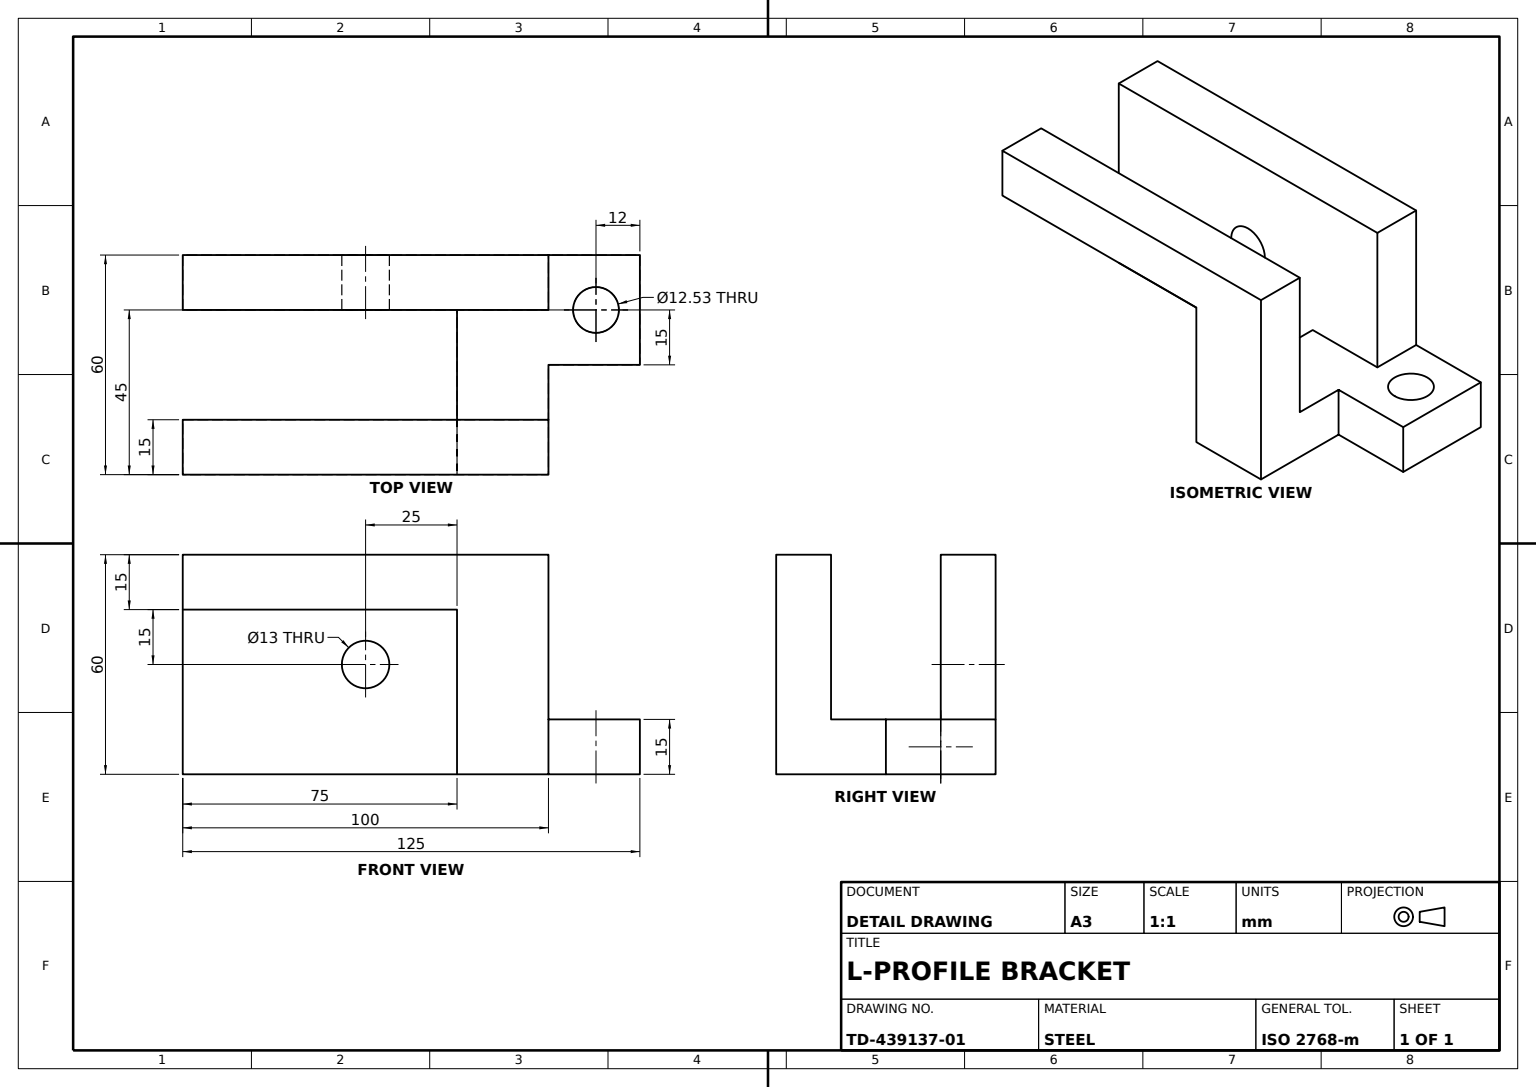
from build123d import *

# Parameters (mm, degrees)
CHANNEL_PROFILE_SKETCH_W = 100
CHANNEL_PROFILE_SKETCH_H = 60
CHANNEL_PROFILE_SKETCH_R = 6.5
CHANNEL_BODY_DEPTH       = 15
LUG_1_PROFILE_SKETCH_R   = 6.266086447
PIERCED_LUG_1_DEPTH      = 15
PIERCED_LUG_2_DEPTH      = 15


with BuildPart() as part:
    # Channel Profile Sketch → Channel Body (new body)
    with BuildSketch(Plane.XY):
        Rectangle(CHANNEL_PROFILE_SKETCH_W, CHANNEL_PROFILE_SKETCH_H)
        Circle(CHANNEL_PROFILE_SKETCH_R, mode=Mode.SUBTRACT)
    extrude(amount=CHANNEL_BODY_DEPTH)

    # Lug 1 Profile Sketch → Pierced Lug 1 (add)
    with BuildSketch(Plane.XZ.offset(30)):
        Polygon((25, 0), (75, 0), (75, 30), (50, 30), (50, 60), (25, 60), align=None)
        with Locations(Location((63, 15, 0), (0, 0, 270))):
            Circle(LUG_1_PROFILE_SKETCH_R, mode=Mode.SUBTRACT)
    extrude(amount=-PIERCED_LUG_1_DEPTH)

    # Lug 2 Profile Sketch → Pierced Lug 2 (add)
    with BuildSketch(Plane.XY.offset(60)):
        Polygon((25, -30), (50, -30), (50, 30), (-50, 30), (-50, 15), (25, 15), align=None)
    extrude(amount=-PIERCED_LUG_2_DEPTH)


solid = part.part
